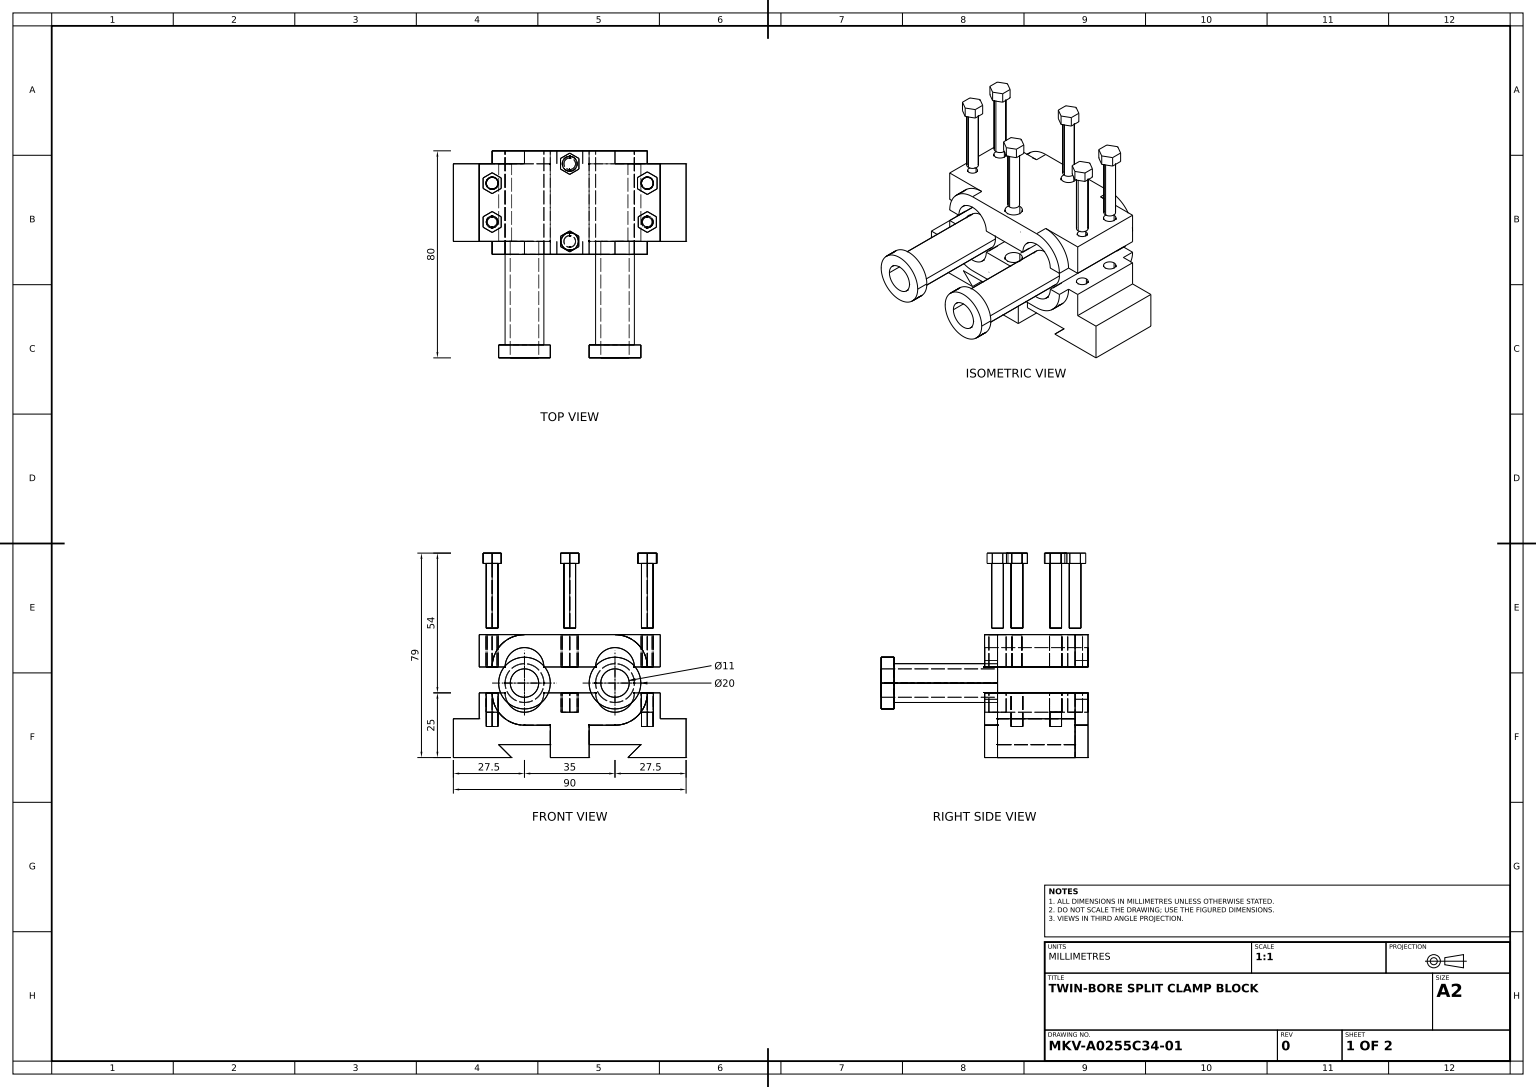
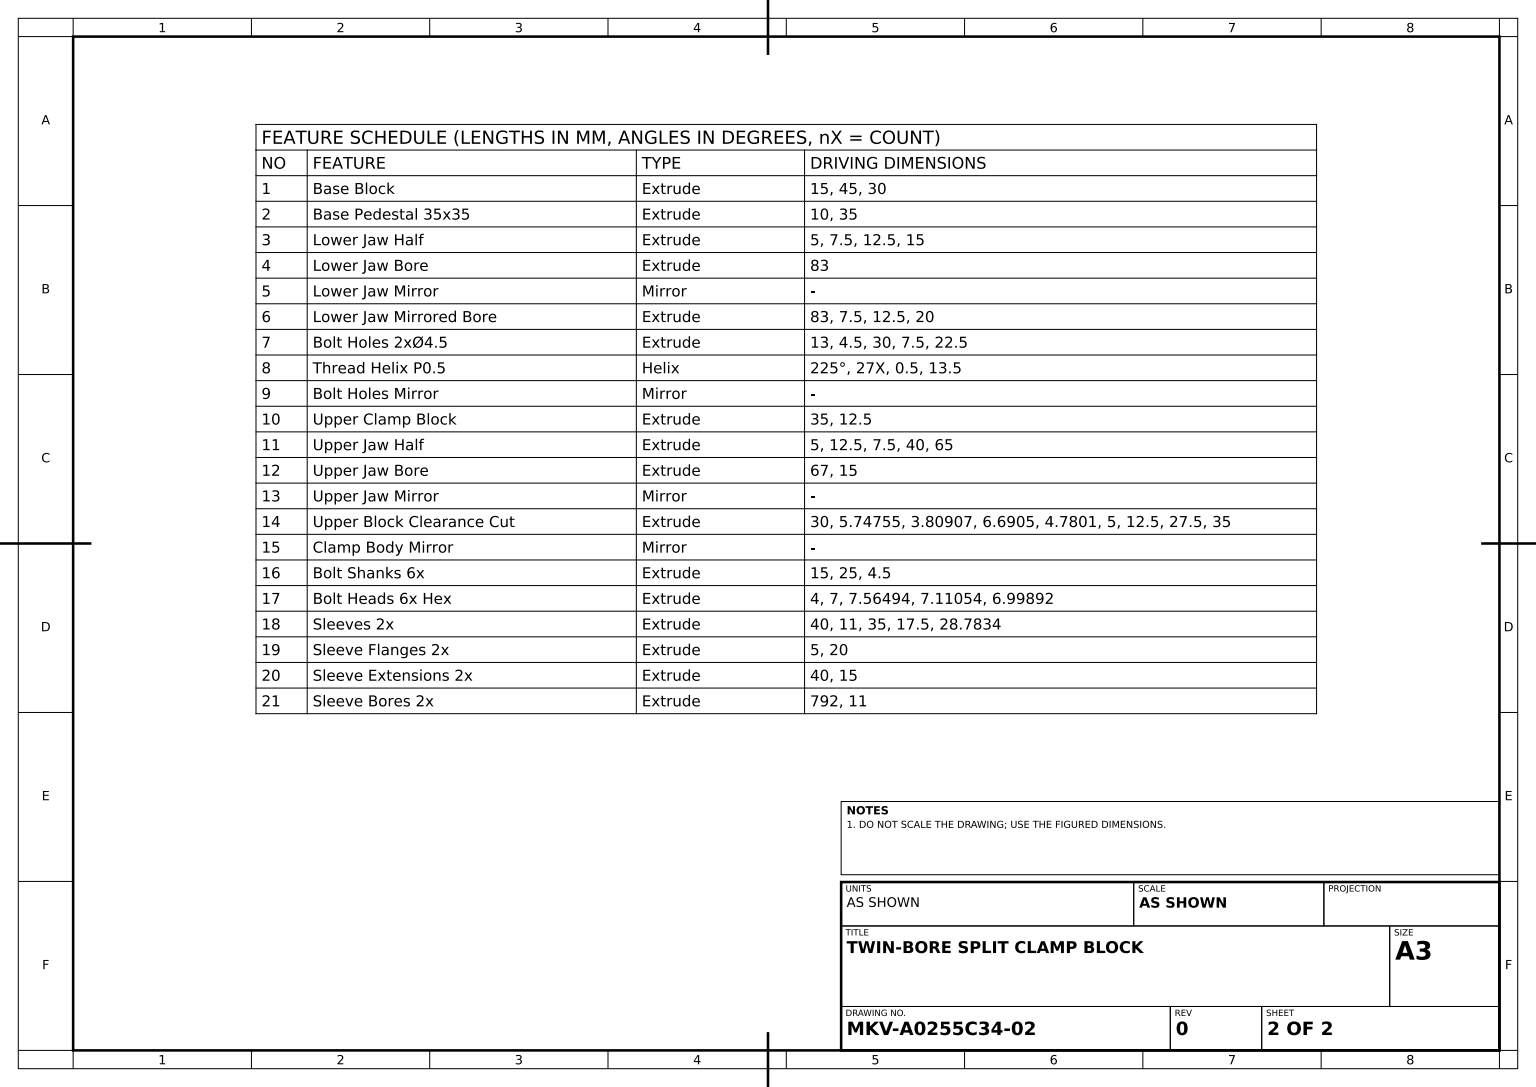
from build123d import *

# Parameters (mm, degrees)
BASE_BLOCK_DEPTH                 = 15
BASE_PEDESTAL_SKETCH_W           = 70
BASE_PEDESTAL_SKETCH_H           = 30
BASE_PEDESTAL_35X35_DEPTH        = 10
LOWER_JAW_HALF_DEPTH             = 5
LOWER_START                      = -83
LOWER_JAW_BORE_SKETCH_R          = 7.5
LOWER_JAW_BORE_DEPTH             = 83
LOWER_JAW_MIRRORED_BORE_DEPTH    = 83
BOLT_HOLES_SKETCH_R              = 2.25
BOLT_HOLES_2X_4_5_DEPTH          = 13
UPPER_CLAMP_BLOCK_SKETCH_W       = 70
UPPER_CLAMP_BLOCK_SKETCH_H       = 30
UPPER_CLAMP_BLOCK_DEPTH          = 12.5
UPPER_JAW_HALF_DEPTH             = 5
UPPER_JAW_BORE_SKETCH_R          = 7.5
UPPER_JAW_BORE_DEPTH             = 67
UPPER_BLOCK_CLEARANCE_SKETCH_R   = 2.390051805
UPPER_BLOCK_CLEARANCE_SKETCH_R_2 = 1.904536549
UPPER_BLOCK_CLEARANCE_SKETCH_R_3 = 2.873773491
UPPER_BLOCK_CLEARANCE_SKETCH_R_4 = 3.345251954
UPPER_BLOCK_CLEARANCE_CUT_DEPTH  = 30
BOLT_SHANKS_SKETCH_R             = 2.25
BOLT_SHANKS_6X_DEPTH             = 25
BOLT_SHANKS_6X_2_DEPTH           = 25
BOLT_SHANKS_6X_3_DEPTH           = 25
BOLT_SHANKS_6X_4_DEPTH           = 25
BOLT_SHANKS_6X_5_DEPTH           = 25
BOLT_SHANKS_6X_6_DEPTH           = 25
BOLT_HEADS_6X_HEX_DEPTH          = 4
SLEEVES_SKETCH_R                 = 5.5
SLEEVES_2X_DEPTH                 = 40
SLEEVES_2X_2_DEPTH               = 40
SLEEVE_FLANGES_SKETCH_R          = 10
SLEEVE_FLANGES_2X_DEPTH          = 5
SLEEVE_EXTENSIONS_SKETCH_R       = 7.5
SLEEVE_EXTENSIONS_2X_DEPTH       = 40
SLEEVE_BORES_SKETCH_R            = 5.5
SLEEVE_BORES_2X_DEPTH            = 792


with BuildPart() as part:
    # Base Block Sketch → Base Block (new body)
    with BuildSketch(Plane(origin=(0, 0, 0), x_dir=(1, 0, 0), z_dir=(0, 1, 0))):
        Polygon((0, 0), (45, 0), (45, 30), (-45, 30), (-45, 0), align=None)
    extrude(amount=BASE_BLOCK_DEPTH)

    # Base Pedestal Sketch → Base Pedestal 35x35 (add)
    with BuildSketch(Plane(origin=(0, 15, 0), x_dir=(1, 0, 0), z_dir=(0, 1, 0))):
        with Locations((0, 15)):
            Rectangle(BASE_PEDESTAL_SKETCH_W, BASE_PEDESTAL_SKETCH_H)
    extrude(amount=BASE_PEDESTAL_35X35_DEPTH)

    # Lower Jaw Sketch → Lower Jaw Half (add)
    with BuildSketch(Plane.XY):
        with BuildLine():
            Line((-25, 25), (-30, 25))
            ThreePointArc((-30, 25), (-26.338834765, 16.161165235), (-17.5, 12.5))
            Line((-17.5, 12.5), (-7.5, 12.5))
            Line((-7.5, 12.5), (-7.5, 0))
            Line((-7.5, 0), (0, 0))
            Line((0, 0), (7.5, 0))
            Line((7.5, 0), (7.5, 12.5))
            Line((7.5, 12.5), (17.5, 12.5))
            ThreePointArc((17.5, 12.5), (26.338834765, 16.161165235), (30, 25))
            Line((30, 25), (25, 25))
            ThreePointArc((25, 25), (17.5, 17.5), (10, 25))
            Line((10, 25), (-10, 25))
            ThreePointArc((-10, 25), (-17.5, 17.5), (-25, 25))
        make_face()
    lower_jaw_half = extrude(amount=LOWER_JAW_HALF_DEPTH)

    # Lower Jaw Bore Sketch → Lower Jaw Bore (cut)
    with BuildSketch(Plane.XY.offset(5).offset(LOWER_START)):
        with Locations((-17.5, 25)):
            Circle(LOWER_JAW_BORE_SKETCH_R)
        with Locations((17.5, 25)):
            Circle(LOWER_JAW_BORE_SKETCH_R)
    extrude(amount=LOWER_JAW_BORE_DEPTH, mode=Mode.SUBTRACT)

    # Lower Jaw Mirror: Lower Jaw Half across plane
    add(lower_jaw_half.mirror(Plane.XY.offset(-15)))

    # Lower Jaw Mirrored Bore Sketch → Lower Jaw Mirrored Bore (cut)
    with BuildSketch(Plane(origin=(0, 0, -30), x_dir=(-1, 0, 0), z_dir=(0, 0, -1))):
        Polygon((-27.5, 5), (-22.5, 0), (-7.5, 0), (-7.5, 5), align=None)
        Polygon((7.5, 5), (7.5, 0), (22.5, 0), (27.5, 5), align=None)
    extrude(amount=-LOWER_JAW_MIRRORED_BORE_DEPTH, mode=Mode.SUBTRACT)

    # Bolt Holes Sketch → Bolt Holes 2xØ4.5 (cut)
    with BuildSketch(Plane(origin=(0, 25, 0), x_dir=(1, 0, 0), z_dir=(0, 1, 0))):
        with Locations(Location((30, 7.5, 0), (0, 0, 270))):
            Circle(BOLT_HOLES_SKETCH_R)
        with Locations(Location((30, 22.5, 0), (0, 0, 270))):
            Circle(BOLT_HOLES_SKETCH_R)
    bolt_holes_2x_4_5 = extrude(amount=-BOLT_HOLES_2X_4_5_DEPTH, mode=Mode.SUBTRACT)

    # Bolt Holes Mirror: Bolt Holes 2xØ4.5 across plane
    add(bolt_holes_2x_4_5.mirror(Plane(origin=(0, 0, 0), x_dir=(0, 0, 1), z_dir=(1, 0, 0))), mode=Mode.SUBTRACT)


with BuildPart() as body_2:
    # Upper Clamp Block Sketch → Upper Clamp Block (new body)
    with BuildSketch(Plane(origin=(0, 35, 0), x_dir=(1, 0, 0), z_dir=(0, 1, 0))):
        with Locations((0, 15)):
            Rectangle(UPPER_CLAMP_BLOCK_SKETCH_W, UPPER_CLAMP_BLOCK_SKETCH_H)
    extrude(amount=UPPER_CLAMP_BLOCK_DEPTH)

    # Upper Jaw Sketch → Upper Jaw Half (add)
    with BuildSketch(Plane.XY):
        with BuildLine():
            ThreePointArc((-17.5, 47.5), (-26.338834765, 43.838834765), (-30, 35))
            Line((-30, 35), (-25, 35))
            ThreePointArc((-25, 35), (-17.5, 42.5), (-10, 35))
            Line((-10, 35), (-5, 35))
            Line((-5, 35), (5, 35))
            Line((5, 35), (10, 35))
            ThreePointArc((10, 35), (17.5, 42.5), (25, 35))
            Line((25, 35), (30, 35))
            ThreePointArc((30, 35), (26.338834765, 43.838834765), (17.5, 47.5))
            Line((17.5, 47.5), (-17.5, 47.5))
        make_face()
    upper_jaw_half = extrude(amount=UPPER_JAW_HALF_DEPTH)

    # Upper Jaw Bore Sketch → Upper Jaw Bore (cut)
    with BuildSketch(Plane.XY.offset(5)):
        with Locations((-17.5, 35)):
            Circle(UPPER_JAW_BORE_SKETCH_R)
        with Locations((17.5, 35)):
            Circle(UPPER_JAW_BORE_SKETCH_R)
    extrude(amount=-UPPER_JAW_BORE_DEPTH, mode=Mode.SUBTRACT)

    # Upper Jaw Mirror: Upper Jaw Half across plane
    add(upper_jaw_half.mirror(Plane.XY.offset(-15)))


with BuildPart() as upper_block_clearance_cut_tool:
    # Upper Block Clearance Sketch → Upper Block Clearance Cut (new body)
    with BuildSketch(Plane(origin=(0, 47.5, 0), x_dir=(1, 0, 0), z_dir=(0, 1, 0))):
        with Locations(Location((30, 22.5, 0), (0, 0, 270))):
            Circle(UPPER_BLOCK_CLEARANCE_SKETCH_R)
        with Locations(Location((30, 7.5, 0), (0, 0, 270))):
            Circle(UPPER_BLOCK_CLEARANCE_SKETCH_R_2)
        with Locations(Location((0, 30, 0), (0, 0, 270))):
            Circle(UPPER_BLOCK_CLEARANCE_SKETCH_R_3)
        with Locations(Location((0, 0, 0), (0, 0, 270))):
            Circle(UPPER_BLOCK_CLEARANCE_SKETCH_R_4)
    upper_block_clearance_cut = extrude(amount=-UPPER_BLOCK_CLEARANCE_CUT_DEPTH)


with BuildPart() as part_1:
    add(part.part)

    # Upper Block Clearance Cut: cut by upper_block_clearance_cut_tool
    add(upper_block_clearance_cut_tool.part, mode=Mode.SUBTRACT)


with BuildPart() as body_2_1:
    add(body_2.part)

    # Upper Block Clearance Cut: cut by upper_block_clearance_cut_tool
    add(upper_block_clearance_cut_tool.part, mode=Mode.SUBTRACT)


with BuildPart() as clamp_body_mirror_tool:
    # Clamp Body Mirror: Upper Block Clearance Cut across plane
    add(upper_block_clearance_cut.mirror(Plane(origin=(0, 0, 0), x_dir=(0, 0, 1), z_dir=(1, 0, 0))))


with BuildPart() as part_2:
    add(part_1.part)

    # Clamp Body Mirror: cut by clamp_body_mirror_tool
    add(clamp_body_mirror_tool.part, mode=Mode.SUBTRACT)


with BuildPart() as body_2_2:
    add(body_2_1.part)

    # Clamp Body Mirror: cut by clamp_body_mirror_tool
    add(clamp_body_mirror_tool.part, mode=Mode.SUBTRACT)


with BuildPart() as body_3:
    # Bolt Shanks Sketch → Bolt Shanks 6x (new body)
    with BuildSketch(Plane(origin=(0, 50, 0), x_dir=(1, 0, 0), z_dir=(0, 1, 0))):
        with Locations(Location((0, 0, 0), (0, 0, 270))):
            Circle(BOLT_SHANKS_SKETCH_R)
    extrude(amount=BOLT_SHANKS_6X_DEPTH)



with BuildPart() as body_4:
    # Bolt Shanks Sketch → Bolt Shanks 6x 2 (new body)
    with BuildSketch(Plane(origin=(0, 50, 0), x_dir=(1, 0, 0), z_dir=(0, 1, 0))):
        with Locations(Location((30, 22.5, 0), (0, 0, 270))):
            Circle(BOLT_SHANKS_SKETCH_R)
    extrude(amount=BOLT_SHANKS_6X_2_DEPTH)


with BuildPart() as body_5:
    # Bolt Shanks Sketch → Bolt Shanks 6x 3 (new body)
    with BuildSketch(Plane(origin=(0, 50, 0), x_dir=(1, 0, 0), z_dir=(0, 1, 0))):
        with Locations(Location((30, 7.5, 0), (0, 0, 270))):
            Circle(BOLT_SHANKS_SKETCH_R)
    extrude(amount=BOLT_SHANKS_6X_3_DEPTH)


with BuildPart() as body_6:
    # Bolt Shanks Sketch → Bolt Shanks 6x 4 (new body)
    with BuildSketch(Plane(origin=(0, 50, 0), x_dir=(1, 0, 0), z_dir=(0, 1, 0))):
        with Locations(Location((0, 30, 0), (0, 0, 270))):
            Circle(BOLT_SHANKS_SKETCH_R)
    extrude(amount=BOLT_SHANKS_6X_4_DEPTH)


with BuildPart() as body_7:
    # Bolt Shanks Sketch → Bolt Shanks 6x 5 (new body)
    with BuildSketch(Plane(origin=(0, 50, 0), x_dir=(1, 0, 0), z_dir=(0, 1, 0))):
        with Locations(Location((-30, 7.5, 0), (0, 0, 270))):
            Circle(BOLT_SHANKS_SKETCH_R)
    extrude(amount=BOLT_SHANKS_6X_5_DEPTH)


with BuildPart() as body_8:
    # Bolt Shanks Sketch → Bolt Shanks 6x 6 (new body)
    with BuildSketch(Plane(origin=(0, 50, 0), x_dir=(1, 0, 0), z_dir=(0, 1, 0))):
        with Locations(Location((-30, 22.5, 0), (0, 0, 270))):
            Circle(BOLT_SHANKS_SKETCH_R)
    extrude(amount=BOLT_SHANKS_6X_6_DEPTH)


with BuildPart() as body_3_1:
    add(body_3.part)

    add(body_4.part)  # Bolt Heads 6x Hex merges body 4

    add(body_5.part)  # Bolt Heads 6x Hex merges body 5

    add(body_6.part)  # Bolt Heads 6x Hex merges body 6

    add(body_7.part)  # Bolt Heads 6x Hex merges body 7

    add(body_8.part)  # Bolt Heads 6x Hex merges body 8
    # Bolt Heads Sketch → Bolt Heads 6x Hex (add)
    with BuildSketch(Plane(origin=(0, 75, 0), x_dir=(1, 0, 0), z_dir=(0, 1, 0))):
        Polygon((0, 34.105271911), (-3.555269764, 32.052635955), (-3.555269764, 27.947364045), (0, 25.894728089), (3.555269764, 27.947364045), (3.555269764, 32.052635955), align=None)
        Polygon((0, 4.041451884), (-3.5, 2.020725942), (-3.5, -2.020725942), (0, -4.041451884), (3.5, -2.020725942), (3.5, 2.020725942), align=None)
        Polygon((30, 26.867620156), (26.217529991, 24.683810078), (26.217529991, 20.316189922), (30, 18.132379844), (33.782470009, 20.316189922), (33.782470009, 24.683810078), align=None)
        Polygon((30, 11.540828206), (26.500540122, 9.520414103), (26.500540122, 5.479585897), (30, 3.459171794), (33.499459878, 5.479585897), (33.499459878, 9.520414103), align=None)
        Polygon((-30, 26.541451884), (-33.5, 24.520725942), (-33.5, 20.479274058), (-30, 18.458548116), (-26.5, 20.479274058), (-26.5, 24.520725942), align=None)
        Polygon((-30, 11.541451884), (-33.5, 9.520725942), (-33.5, 5.479274058), (-30, 3.458548116), (-26.5, 5.479274058), (-26.5, 9.520725942), align=None)
    extrude(amount=BOLT_HEADS_6X_HEX_DEPTH)


with BuildPart() as body_4_2:
    # Sleeves Sketch → Sleeves 2x (new body)
    with BuildSketch(Plane.XY):
        with Locations((-17.5, 28.783350127)):
            Circle(SLEEVES_SKETCH_R)
    extrude(amount=SLEEVES_2X_DEPTH)



with BuildPart() as body_5_2:
    # Sleeves Sketch → Sleeves 2x 2 (new body)
    with BuildSketch(Plane.XY):
        with Locations((17.5, 28.783350127)):
            Circle(SLEEVES_SKETCH_R)
    extrude(amount=SLEEVES_2X_2_DEPTH)


with BuildPart() as body_4_2_1:
    add(body_4_2.part)

    add(body_5_2.part)  # Sleeve Flanges 2x merges body 5 2
    # Sleeve Flanges Sketch → Sleeve Flanges 2x (add)
    with BuildSketch(Plane.XY.offset(40)):
        with Locations((-17.5, 28.783350127)):
            Circle(SLEEVE_FLANGES_SKETCH_R)
        with Locations((17.5, 28.783350127)):
            Circle(SLEEVE_FLANGES_SKETCH_R)
    extrude(amount=SLEEVE_FLANGES_2X_DEPTH)

    # Sleeve Extensions Sketch → Sleeve Extensions 2x (add)
    with BuildSketch(Plane(origin=(0, 0, 0), x_dir=(-1, 0, 0), z_dir=(0, 0, -1))):
        with Locations((-17.5, 28.783350127)):
            Circle(SLEEVE_EXTENSIONS_SKETCH_R)
        with Locations((17.5, 28.783350127)):
            Circle(SLEEVE_EXTENSIONS_SKETCH_R)
    extrude(amount=-SLEEVE_EXTENSIONS_2X_DEPTH)

    # Sleeve Bores Sketch → Sleeve Bores 2x (cut)
    with BuildSketch(Plane.XY.offset(45)):
        with Locations((-17.5, 28.783350127)):
            Circle(SLEEVE_BORES_SKETCH_R)
        with Locations((17.5, 28.783350127)):
            Circle(SLEEVE_BORES_SKETCH_R)
    extrude(amount=-SLEEVE_BORES_2X_DEPTH, mode=Mode.SUBTRACT)


solid = Compound([part_2.part, body_2_2.part, body_3_1.part, body_4_2_1.part])
